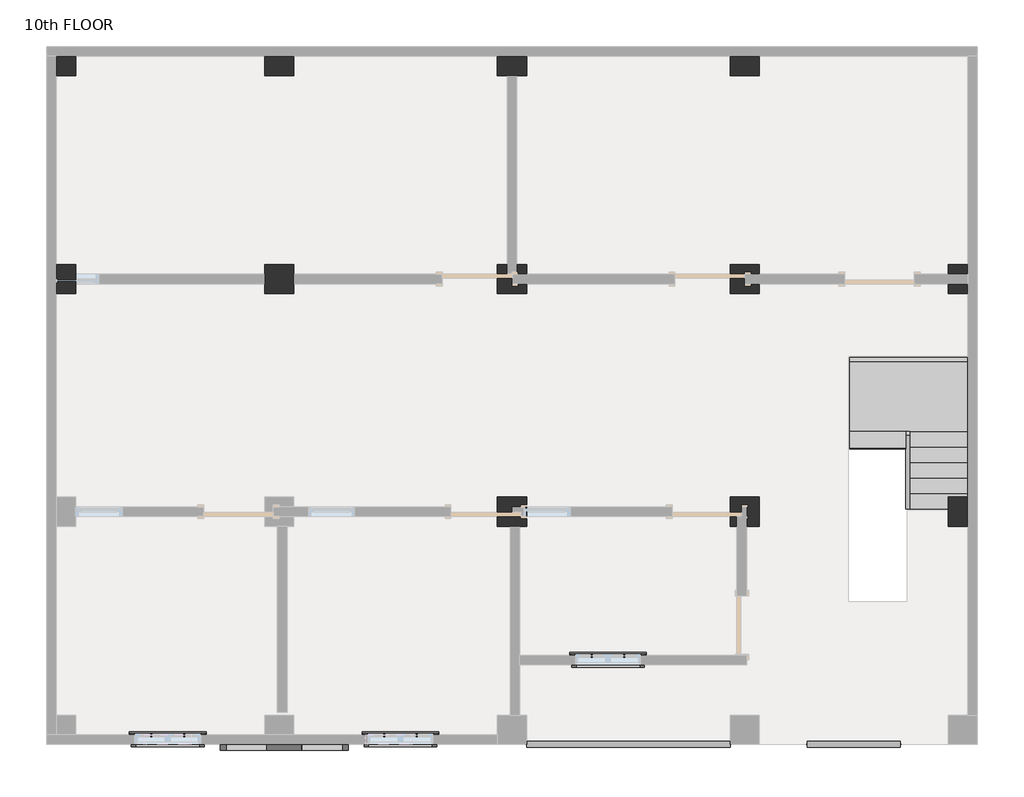
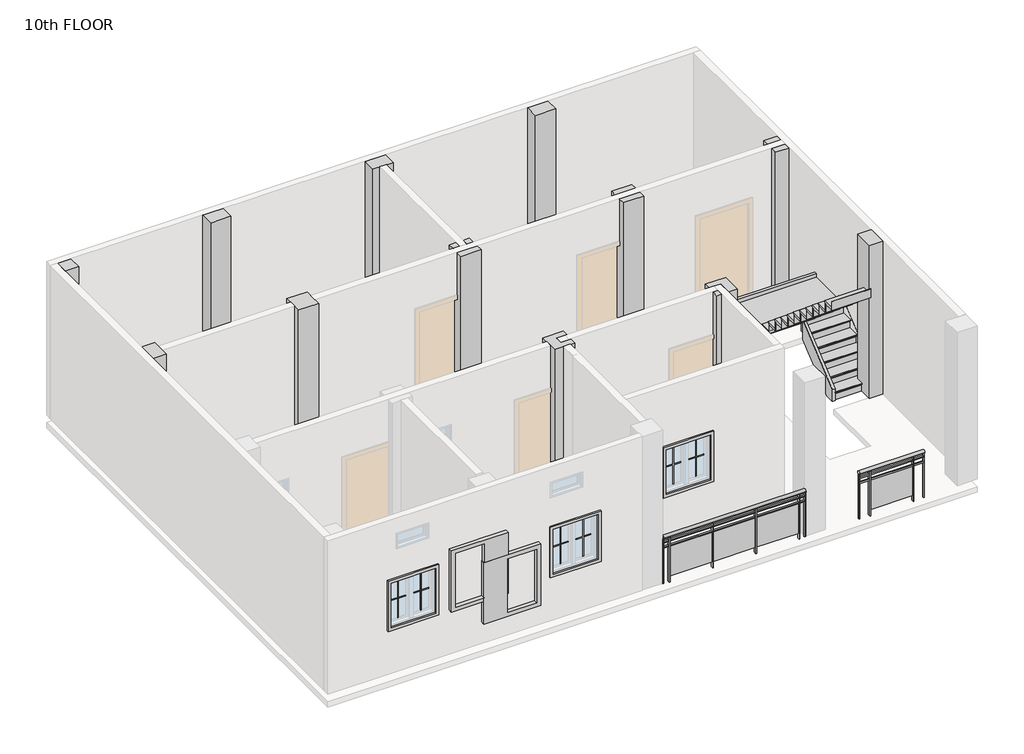
# One storey, part 2 of 2: 12 columns, 12 proxies, 4 members, 2 railings, 1 damper, 1 stair flight.
"""IFC4 building model written with IfcOpenShell, lengths in millimetres."""

from ifc_helpers import new_model, si_unit, point, frame, origin, place, context, project, spatial, polyline, ellipse_curve, trimmed, outline, extrude, faceted_brep, transform, mapped, element, save
from ifc_brep_helpers import plane_surface, extruded_surface, advanced_brep
from components import muntin_pattern_2x2_muntin_pattern_2x2_b3fe6957, muntin_pattern_2x2_muntin_pattern_2x2_3e0ecaf2, trim_window_exterior_flat_with_sill_41619996, trim_window_interior_flat_picture_frame_51c85655, duct_accessories_3_duct_accessories_1_969fcb05, stair_flight_e7bd6350

model = new_model("IFC4")

# Units and contexts
model_context = context("Model", 3, world=origin())
ifc_project = project(units=[si_unit("LENGTHUNIT", "METRE", prefix="MILLI")], contexts=[model_context])

# Site, building, storey
site = spatial("IfcSite", under=ifc_project)
building = spatial("IfcBuilding", under=site)
storey = spatial("IfcBuildingStorey", under=building, Name="10th FLOOR", Elevation=30327.6)

# Proxies
placement = place(None, origin())
muntin_pattern_2x2_muntin_pattern_2x2_shape = muntin_pattern_2x2_muntin_pattern_2x2_b3fe6957(model_context)
element("IfcBuildingElementProxy", 1, Name="Muntin Pattern_2x2 : Muntin Pattern_2x2", ObjectType="Muntin Pattern_2x2 : Muntin Pattern_2x2", at=placement, inside=storey, context=model_context, shape_type="MappedRepresentation", body=[
    mapped(muntin_pattern_2x2_muntin_pattern_2x2_shape, transform((-14441.409625, -253.8184478, 31311.85), x_axis=(1.0, 0.0, 0.0), y_axis=(0.0, 1.0, 0.0), z_axis=(0.0, 0.0, 1.0))),
])
element("IfcBuildingElementProxy", 2, Name="Muntin Pattern_2x2 : Muntin Pattern_2x2", ObjectType="Muntin Pattern_2x2 : Muntin Pattern_2x2", at=placement, inside=storey, context=model_context, shape_type="MappedRepresentation", body=[
    mapped(muntin_pattern_2x2_muntin_pattern_2x2_shape, transform((-11393.409625, -253.8184478, 31311.85), x_axis=(1.0, 0.0, 0.0), y_axis=(0.0, 1.0, 0.0), z_axis=(0.0, 0.0, 1.0))),
])
element("IfcBuildingElementProxy", 3, Name="Muntin Pattern_2x2 : Muntin Pattern_2x2", ObjectType="Muntin Pattern_2x2 : Muntin Pattern_2x2", at=placement, inside=storey, context=model_context, shape_type="MappedRepresentation", body=[
    mapped(muntin_pattern_2x2_muntin_pattern_2x2_shape, transform((-8675.609625, 787.5815522, 31311.85), x_axis=(1.0, 0.0, 0.0), y_axis=(0.0, 1.0, 0.0), z_axis=(0.0, 0.0, 1.0))),
])
muntin_pattern_2x2_muntin_pattern_2x2_2_shape = muntin_pattern_2x2_muntin_pattern_2x2_3e0ecaf2(model_context)
element("IfcBuildingElementProxy", 4, Name="Muntin Pattern_2x2 : Muntin Pattern_2x2", ObjectType="Muntin Pattern_2x2 : Muntin Pattern_2x2", at=placement, inside=storey, context=model_context, shape_type="MappedRepresentation", body=[
    mapped(muntin_pattern_2x2_muntin_pattern_2x2_2_shape, transform((-14012.784625, -253.8184478, 31311.85), x_axis=(-1.0, 0.0, 0.0), y_axis=(0.0, -1.0, 0.0), z_axis=(0.0, 0.0, 1.0))),
])
element("IfcBuildingElementProxy", 5, Name="Muntin Pattern_2x2 : Muntin Pattern_2x2", ObjectType="Muntin Pattern_2x2 : Muntin Pattern_2x2", at=placement, inside=storey, context=model_context, shape_type="MappedRepresentation", body=[
    mapped(muntin_pattern_2x2_muntin_pattern_2x2_2_shape, transform((-10964.784625, -253.8184478, 31311.85), x_axis=(-1.0, 0.0, 0.0), y_axis=(0.0, -1.0, 0.0), z_axis=(0.0, 0.0, 1.0))),
])
element("IfcBuildingElementProxy", 6, Name="Muntin Pattern_2x2 : Muntin Pattern_2x2", ObjectType="Muntin Pattern_2x2 : Muntin Pattern_2x2", at=placement, inside=storey, context=model_context, shape_type="MappedRepresentation", body=[
    mapped(muntin_pattern_2x2_muntin_pattern_2x2_2_shape, transform((-8246.984625, 787.5815522, 31311.85), x_axis=(-1.0, 0.0, 0.0), y_axis=(0.0, -1.0, 0.0), z_axis=(0.0, 0.0, 1.0))),
])
trim_window_exterior_flat_with_sill_shape = trim_window_exterior_flat_with_sill_41619996(model_context)
element("IfcBuildingElementProxy", 7, Name="Trim-Window-Exterior-Flat : with Sill", ObjectType="Trim-Window-Exterior-Flat : with Sill", at=placement, inside=storey, context=model_context, shape_type="MappedRepresentation", body=[
    mapped(trim_window_exterior_flat_with_sill_shape, transform((-14227.097125, -244.2934478, 32156.4), x_axis=(-1.0, 0.0, 0.0), y_axis=(0.0, 0.0, 1.0), z_axis=(0.0, 1.0, 0.0))),
])
element("IfcBuildingElementProxy", 8, Name="Trim-Window-Exterior-Flat : with Sill", ObjectType="Trim-Window-Exterior-Flat : with Sill", at=placement, inside=storey, context=model_context, shape_type="MappedRepresentation", body=[
    mapped(trim_window_exterior_flat_with_sill_shape, transform((-11179.097125, -244.2934478, 32156.4), x_axis=(-1.0, 0.0, 0.0), y_axis=(0.0, 0.0, 1.0), z_axis=(0.0, 1.0, 0.0))),
])
element("IfcBuildingElementProxy", 9, Name="Trim-Window-Exterior-Flat : with Sill", ObjectType="Trim-Window-Exterior-Flat : with Sill", at=placement, inside=storey, context=model_context, shape_type="MappedRepresentation", body=[
    mapped(trim_window_exterior_flat_with_sill_shape, transform((-8461.297125, 797.1065522, 32156.4), x_axis=(-1.0, 0.0, 0.0), y_axis=(0.0, 0.0, 1.0), z_axis=(0.0, 1.0, 0.0))),
])
trim_window_interior_flat_picture_frame_shape = trim_window_interior_flat_picture_frame_51c85655(model_context)
element("IfcBuildingElementProxy", 10, Name="Trim-Window-Interior-Flat : Picture Frame", ObjectType="Trim-Window-Interior-Flat : Picture Frame", at=placement, inside=storey, context=model_context, shape_type="MappedRepresentation", body=[
    mapped(trim_window_interior_flat_picture_frame_shape, transform((-14227.097125, -371.2934478, 32156.4), x_axis=(1.0, 0.0, 0.0), y_axis=(0.0, 0.0, 1.0), z_axis=(0.0, -1.0, 0.0))),
])
element("IfcBuildingElementProxy", 11, Name="Trim-Window-Interior-Flat : Picture Frame", ObjectType="Trim-Window-Interior-Flat : Picture Frame", at=placement, inside=storey, context=model_context, shape_type="MappedRepresentation", body=[
    mapped(trim_window_interior_flat_picture_frame_shape, transform((-11179.097125, -371.2934478, 32156.4), x_axis=(1.0, 0.0, 0.0), y_axis=(0.0, 0.0, 1.0), z_axis=(0.0, -1.0, 0.0))),
])
element("IfcBuildingElementProxy", 12, Name="Trim-Window-Interior-Flat : Picture Frame", ObjectType="Trim-Window-Interior-Flat : Picture Frame", at=placement, inside=storey, context=model_context, shape_type="MappedRepresentation", body=[
    mapped(trim_window_interior_flat_picture_frame_shape, transform((-8461.297125, 670.1065522, 32156.4), x_axis=(1.0, 0.0, 0.0), y_axis=(0.0, 0.0, 1.0), z_axis=(0.0, -1.0, 0.0))),
])

# Columns
element("IfcColumn", 13, ObjectType="column family : column family", at=placement, inside=storey, context=model_context, shape_type="SweptSolid", body=[
    extrude(outline(polyline([(-15433.597125, 8645.7065522), (-15433.597125, 8391.7065522), (-15687.597125, 8391.7065522), (-15687.597125, 8645.7065522), (-15433.597125, 8645.7065522)])), frame((0.0, 0.0, 30332.6), z_axis=(0.0, 0.0, 1.0), x_axis=(1.0, 0.0, 0.0)), (0.0, 0.0, 1.0), 3038.0),
])
element("IfcColumn", 14, ObjectType="column family : column family", at=placement, inside=storey, context=model_context, shape_type="SweptSolid", body=[
    extrude(outline(polyline([(-12576.097125, 5915.2065522), (-12576.097125, 5534.2065522), (-12957.097125, 5534.2065522), (-12957.097125, 5915.2065522), (-12576.097125, 5915.2065522)])), frame((0.0, 0.0, 30332.6), z_axis=(0.0, 0.0, 1.0), x_axis=(1.0, 0.0, 0.0)), (0.0, 0.0, 1.0), 3038.0),
])
element("IfcColumn", 15, ObjectType="column family : column family", at=placement, inside=storey, context=model_context, shape_type="Brep", body=[
    faceted_brep([(-9655.097125, 5915.2065522, 30332.6), (-9528.097125, 5915.2065522, 30332.6), (-9528.097125, 5788.2065522, 30332.6), (-9655.097125, 5788.2065522, 30332.6), (-9528.097125, 5915.2065522, 33370.6), (-9655.097125, 5915.2065522, 33370.6), (-9655.097125, 5788.2065522, 33370.6), (-9528.097125, 5788.2065522, 33370.6)], [[[0, 1, 2, 3]], [[4, 5, 6, 7]], [[0, 3, 6, 5]], [[4, 1, 0, 5]], [[3, 2, 7, 6]], [[1, 4, 7, 2]]]),
    faceted_brep([(-9528.097125, 5534.2065522, 33370.6), (-9528.097125, 5534.2065522, 30332.6), (-9528.097125, 5661.2065522, 30332.6), (-9528.097125, 5661.2065522, 33370.6), (-9909.097125, 5534.2065522, 30332.6), (-9909.097125, 5534.2065522, 33370.6), (-9909.097125, 5915.2065522, 30332.6), (-9909.097125, 5661.2065522, 33370.6), (-9909.097125, 5661.2065522, 32461.2), (-9909.097125, 5788.2065522, 32461.2), (-9909.097125, 5788.2065522, 33370.6), (-9909.097125, 5915.2065522, 33370.6), (-9782.097125, 5915.2065522, 33370.6), (-9782.097125, 5915.2065522, 30332.6), (-9782.097125, 5788.2065522, 30332.6), (-9782.097125, 5788.2065522, 33370.6), (-9782.097125, 5788.2065522, 32461.2), (-9718.597125, 5788.2065522, 30332.6), (-9718.597125, 5788.2065522, 32461.2), (-9718.597125, 5661.2065522, 30332.6), (-9718.597125, 5661.2065522, 32461.2)], [[[0, 1, 2, 3]], [[4, 1, 0, 5]], [[6, 4, 5, 7, 8, 9, 10, 11]], [[6, 11, 12, 13]], [[14, 13, 12, 15, 16]], [[17, 14, 16, 18]], [[19, 20, 8, 7, 3, 2]], [[1, 4, 6, 13, 14, 17, 19, 2]], [[5, 0, 3, 7]], [[12, 11, 10, 15]], [[9, 16, 15, 10]], [[18, 20, 19, 17]], [[20, 18, 16, 9, 8]]]),
])
element("IfcColumn", 16, ObjectType="column family : column family", at=placement, inside=storey, context=model_context, shape_type="Brep", body=[
    faceted_brep([(-6480.097125, 5534.2065522, 30332.6), (-6861.097125, 5534.2065522, 30332.6), (-6861.097125, 5915.2065522, 30332.6), (-6480.097125, 5915.2065522, 30332.6), (-6480.097125, 5788.2065522, 30332.6), (-6670.597125, 5788.2065522, 30332.6), (-6670.597125, 5661.2065522, 30332.6), (-6480.097125, 5661.2065522, 30332.6), (-6480.097125, 5534.2065522, 33370.6), (-6480.097125, 5661.2065522, 33370.6), (-6861.097125, 5534.2065522, 33370.6), (-6861.097125, 5661.2065522, 33370.6), (-6861.097125, 5661.2065522, 32461.2), (-6861.097125, 5788.2065522, 32461.2), (-6861.097125, 5788.2065522, 33370.6), (-6861.097125, 5915.2065522, 33370.6), (-6480.097125, 5915.2065522, 33370.6), (-6670.597125, 5661.2065522, 32461.2), (-6670.597125, 5788.2065522, 32461.2), (-6480.097125, 5788.2065522, 33370.6)], [[[0, 1, 2, 3, 4, 5, 6, 7]], [[8, 0, 7, 9]], [[1, 0, 8, 10]], [[2, 1, 10, 11, 12, 13, 14, 15]], [[3, 2, 15, 16]], [[10, 8, 9, 11]], [[6, 17, 12, 11, 9, 7]], [[13, 18, 5, 4, 19, 14]], [[3, 16, 19, 4]], [[16, 15, 14, 19]], [[18, 17, 6, 5]], [[17, 18, 13, 12]]]),
])
element("IfcColumn", 17, ObjectType="column family : column family", at=placement, inside=storey, context=model_context, shape_type="Brep", body=[
    faceted_brep([(-6480.097125, 2867.2065522, 30332.6), (-6480.097125, 2486.2065522, 30332.6), (-6645.197125, 2486.2065522, 30332.6), (-6645.197125, 2740.2065522, 30332.6), (-6708.697125, 2740.2065522, 30332.6), (-6708.697125, 2613.2065522, 30332.6), (-6772.197125, 2613.2065522, 30332.6), (-6772.197125, 2486.2065522, 30332.6), (-6861.097125, 2486.2065522, 30332.6), (-6861.097125, 2867.2065522, 30332.6), (-6480.097125, 2867.2065522, 33370.6), (-6480.097125, 2486.2065522, 33370.6), (-6861.097125, 2486.2065522, 33370.6), (-6772.197125, 2486.2065522, 33370.6), (-6861.097125, 2613.2065522, 33370.6), (-6861.097125, 2613.2065522, 32461.2), (-6861.097125, 2740.2065522, 32461.2), (-6861.097125, 2740.2065522, 33370.6), (-6861.097125, 2867.2065522, 33370.6), (-6772.197125, 2740.2065522, 33370.6), (-6645.197125, 2740.2065522, 33370.6), (-6645.197125, 2486.2065522, 33370.6), (-6772.197125, 2613.2065522, 33370.6), (-6772.197125, 2613.2065522, 32461.2), (-6772.197125, 2740.2065522, 32461.2), (-6708.697125, 2613.2065522, 32461.2), (-6708.697125, 2740.2065522, 32461.2)], [[[0, 1, 2, 3, 4, 5, 6, 7, 8, 9]], [[1, 0, 10, 11]], [[12, 8, 7, 13]], [[9, 8, 12, 14, 15, 16, 17, 18]], [[0, 9, 18, 10]], [[11, 10, 18, 17, 19, 20, 21]], [[15, 14, 22, 23]], [[17, 16, 24, 19]], [[20, 3, 2, 21]], [[6, 23, 22, 13, 7]], [[14, 12, 13, 22]], [[1, 11, 21, 2]], [[15, 23, 24, 16]], [[25, 23, 6, 5]], [[23, 25, 26, 24]], [[26, 25, 5, 4]], [[24, 26, 4, 3, 20, 19]]]),
])
element("IfcColumn", 18, ObjectType="column family : column family", at=placement, inside=storey, context=model_context, shape_type="Brep", body=[
    faceted_brep([(-9528.097125, 2486.2065522, 30332.6), (-9909.097125, 2486.2065522, 30332.6), (-9909.097125, 2867.2065522, 30332.6), (-9528.097125, 2867.2065522, 30332.6), (-9528.097125, 2740.2065522, 30332.6), (-9566.197125, 2740.2065522, 30332.6), (-9718.597125, 2740.2065522, 30332.6), (-9718.597125, 2613.2065522, 30332.6), (-9566.197125, 2613.2065522, 30332.6), (-9528.097125, 2613.2065522, 30332.6), (-9528.097125, 2486.2065522, 33370.6), (-9528.097125, 2613.2065522, 30632.4), (-9528.097125, 2740.2065522, 30632.4), (-9528.097125, 2867.2065522, 33370.6), (-9528.097125, 2740.2065522, 33370.6), (-9528.097125, 2740.2065522, 32461.2), (-9528.097125, 2613.2065522, 32461.2), (-9528.097125, 2613.2065522, 33370.6), (-9909.097125, 2486.2065522, 33370.6), (-9909.097125, 2867.2065522, 33370.6), (-9566.197125, 2613.2065522, 33370.6), (-9718.597125, 2613.2065522, 33370.6), (-9718.597125, 2740.2065522, 33370.6), (-9566.197125, 2740.2065522, 33370.6), (-9566.197125, 2613.2065522, 32461.2), (-9566.197125, 2613.2065522, 30632.4), (-9566.197125, 2740.2065522, 30632.4), (-9566.197125, 2740.2065522, 32461.2)], [[[0, 1, 2, 3, 4, 5, 6, 7, 8, 9]], [[10, 0, 9, 11, 12, 4, 3, 13, 14, 15, 16, 17]], [[1, 0, 10, 18]], [[2, 1, 18, 19]], [[3, 2, 19, 13]], [[18, 10, 17, 20, 21, 22, 23, 14, 13, 19]], [[11, 9, 8, 7, 21, 20, 17, 16, 24, 25]], [[4, 12, 26, 27, 15, 14, 23, 22, 6, 5]], [[21, 7, 6, 22]], [[25, 24, 27, 26]], [[25, 26, 12, 11]], [[27, 24, 16, 15]]]),
])
element("IfcColumn", 19, ObjectType="column family : column family", at=placement, inside=storey, context=model_context, shape_type="SweptSolid", body=[
    extrude(outline(polyline([(-12576.097125, 8391.7065522), (-12957.097125, 8391.7065522), (-12957.097125, 8645.7065522), (-12576.097125, 8645.7065522), (-12576.097125, 8391.7065522)])), frame((0.0, 0.0, 30332.6), z_axis=(0.0, 0.0, 1.0), x_axis=(1.0, 0.0, 0.0)), (0.0, 0.0, 1.0), 3038.0),
])
element("IfcColumn", 20, ObjectType="column family : column family", at=placement, inside=storey, context=model_context, shape_type="SweptSolid", body=[
    extrude(outline(polyline([(-9528.097125, 8391.7065522), (-9909.097125, 8391.7065522), (-9909.097125, 8645.7065522), (-9528.097125, 8645.7065522), (-9528.097125, 8391.7065522)])), frame((0.0, 0.0, 30332.6), z_axis=(0.0, 0.0, 1.0), x_axis=(1.0, 0.0, 0.0)), (0.0, 0.0, 1.0), 3038.0),
])
element("IfcColumn", 21, ObjectType="column family : column family", at=placement, inside=storey, context=model_context, shape_type="SweptSolid", body=[
    extrude(outline(polyline([(-6480.097125, 8391.7065522), (-6861.097125, 8391.7065522), (-6861.097125, 8645.7065522), (-6480.097125, 8645.7065522), (-6480.097125, 8391.7065522)])), frame((0.0, 0.0, 30332.6), z_axis=(0.0, 0.0, 1.0), x_axis=(1.0, 0.0, 0.0)), (0.0, 0.0, 1.0), 3038.0),
])
element("IfcColumn", 22, ObjectType="column family : column family", at=placement, inside=storey, context=model_context, shape_type="SweptSolid", body=[
    extrude(outline(polyline([(-4003.597125, 5915.2065522), (-3749.597125, 5915.2065522), (-3749.597125, 5788.2065522), (-4003.597125, 5788.2065522), (-4003.597125, 5915.2065522)])), frame((0.0, 0.0, 30332.6), z_axis=(0.0, 0.0, 1.0), x_axis=(1.0, 0.0, 0.0)), (0.0, 0.0, 1.0), 3038.0),
    extrude(outline(polyline([(-3749.597125, 5534.2065522), (-4003.597125, 5534.2065522), (-4003.597125, 5661.2065522), (-3749.597125, 5661.2065522), (-3749.597125, 5534.2065522)])), frame((0.0, 0.0, 30332.6), z_axis=(0.0, 0.0, 1.0), x_axis=(1.0, 0.0, 0.0)), (0.0, 0.0, 1.0), 3038.0),
])
element("IfcColumn", 23, ObjectType="column family : column family", at=placement, inside=storey, context=model_context, shape_type="SweptSolid", body=[
    extrude(outline(polyline([(-4003.597125, 2486.2065522), (-4003.597125, 2867.2065522), (-3749.597125, 2867.2065522), (-3749.597125, 2486.2065522), (-4003.597125, 2486.2065522)])), frame((0.0, 0.0, 30332.6), z_axis=(0.0, 0.0, 1.0), x_axis=(1.0, 0.0, 0.0)), (0.0, 0.0, 1.0), 3038.0),
])
element("IfcColumn", 24, ObjectType="column family : column family", at=placement, inside=storey, context=model_context, shape_type="SweptSolid", body=[
    extrude(outline(polyline([(-15433.597125, 5915.2065522), (-15433.597125, 5534.2065522), (-15687.597125, 5534.2065522), (-15687.597125, 5915.2065522), (-15433.597125, 5915.2065522)])), frame((0.0, 0.0, 30332.6), z_axis=(0.0, 0.0, 1.0), x_axis=(1.0, 0.0, 0.0)), (0.0, 0.0, 1.0), 3038.0),
])

# Damper
duct_accessories_3_duct_accessories_1_shape = duct_accessories_3_duct_accessories_1_969fcb05(model_context)
element("IfcDamper", 25, ObjectType="Duct Accessories 3 : Duct Accessories 1", at=placement, inside=storey, context=model_context, shape_type="MappedRepresentation", body=[
    mapped(duct_accessories_3_duct_accessories_1_shape, transform((0.0, 0.0, 0.0), x_axis=(1.0, 0.0, 0.0), y_axis=(0.0, 1.0, 0.0), z_axis=(0.0, 0.0, 1.0))),
])

# Members
element("IfcMember", 26, ObjectType="Stringer - 2\" Width", at=placement, inside=storey, context=model_context, shape_type="SweptSolid", body=[
    extrude(outline(polyline([(2714.6319226, 30327.6), (2714.6319226, 30564.4438745), (3679.8319226, 31368.7772078), (3679.8319226, 30972.0165243), (2906.5320935, 30327.6), (2714.6319226, 30327.6)])), frame((-4563.0136682, 0.0, 0.0), z_axis=(1.0, 0.0, 0.0), x_axis=(0.0, 1.0, 0.0)), (0.0, 0.0, 1.0), 50.8),
])
element("IfcMember", 27, ObjectType="Stringer - 2\" Width", at=placement, inside=storey, context=model_context, shape_type="SweptSolid", body=[
    extrude(outline(polyline([(-4512.2136682, 3730.6319226), (-4512.2136682, 3679.8319226), (-4563.0136682, 3679.8319226), (-4563.0136682, 3730.6319226), (-4512.2136682, 3730.6319226)])), frame((0.0, 0.0, 31115.0), z_axis=(0.0, 0.0, 1.0), x_axis=(1.0, 0.0, 0.0)), (0.0, 0.0, 1.0), 304.8),
])
element("IfcMember", 28, ObjectType="Stringer - 2\" Width", at=placement, inside=storey, context=model_context, shape_type="SweptSolid", body=[
    extrude(outline(polyline([(2714.6319226, 30327.6), (2714.6319226, 30564.4438745), (3741.0592732, 31419.8), (4217.1720935, 31419.8), (2906.5320935, 30327.6), (2714.6319226, 30327.6)])), frame((-3749.597125, 0.0, 0.0), z_axis=(1.0, 0.0, 0.0), x_axis=(0.0, 1.0, 0.0)), (0.0, 0.0, 1.0), 50.8),
])
element("IfcMember", 29, ObjectType="Stringer - 2\" Width", at=placement, inside=storey, context=model_context, shape_type="SweptSolid", body=[
    extrude(outline(polyline([(-3698.797125, 4695.8319226), (-3698.797125, 4645.0319226), (-5295.0246464, 4645.0319226), (-5295.0246464, 4695.8319226), (-3698.797125, 4695.8319226)])), frame((0.0, 0.0, 31115.0), z_axis=(0.0, 0.0, 1.0), x_axis=(1.0, 0.0, 0.0)), (0.0, 0.0, 1.0), 304.8),
])

# Railings
element("IfcRailing", 30, ObjectType="Glass Panel - Bottom Fill", at=placement, inside=storey, context=model_context, shape_type="SolidModel", body=[
    advanced_brep(
    [(-9528.097125, -333.1934478, 31242.0), (-9528.097125, -409.3934478, 31242.0), (-6861.097125, -333.1934478, 31242.0), (-6861.097125, -409.3934478, 31242.0)],
    [
        (0, 1, ellipse_curve(frame((-9528.097125, -371.2934478, 31242.0), z_axis=(-1.0, 0.0, 0.0), x_axis=(0.0, -1.0, 0.0)), 38.1, 28.575)),
        (1, 0, ellipse_curve(frame((-9528.097125, -371.2934478, 31242.0), z_axis=(-1.0, 0.0, 0.0), x_axis=(0.0, -1.0, 0.0)), 38.1, 28.575)),
        (2, 3, ellipse_curve(frame((-6861.097125, -371.2934478, 31242.0), z_axis=(1.0, 0.0, 0.0), x_axis=(0.0, -1.0, 0.0)), 38.1, 28.575)),
        (3, 2, ellipse_curve(frame((-6861.097125, -371.2934478, 31242.0), z_axis=(1.0, 0.0, 0.0), x_axis=(0.0, -1.0, 0.0)), 38.1, 28.575)),
        (0, 2),
        (3, 1),
    ],
    [
        plane_surface(frame((-9528.097125, -371.2934478, 31242.0), z_axis=(-1.0, 0.0, 0.0), x_axis=(0.0, 1.0, 0.0))),
        plane_surface(frame((-6861.097125, -371.2934478, 31242.0), z_axis=(1.0, 0.0, 0.0), x_axis=(0.0, 1.0, 0.0))),
        extruded_surface(trimmed(ellipse_curve(frame((-6861.097125, -371.2934478, 31242.0), z_axis=(-1.0, 0.0, 0.0), x_axis=(0.0, -1.0, 0.0)), 38.1, 28.575), [point((-6861.097125, -333.1934478, 31242.0))], [point((-6861.097125, -409.3934478, 31242.0))], True, "CARTESIAN"), (-2667.0, 0.0, 0.0), 2667.0),
        extruded_surface(trimmed(ellipse_curve(frame((-6861.097125, -371.2934478, 31242.0), z_axis=(-1.0, 0.0, 0.0), x_axis=(0.0, -1.0, 0.0)), 38.1, 28.575), [point((-6861.097125, -409.3934478, 31242.0))], [point((-6861.097125, -333.1934478, 31242.0))], True, "CARTESIAN"), (-2667.0, 0.0, 0.0), 2667.0),
    ],
    [
        (0, [[1, 2]]),
        (1, [[3, 4]]),
        (2, [[-1, 5, -4, 6]]),
        (3, [[-2, -6, -3, -5]]),
    ],
),
    extrude(outline(polyline([(-9528.097125, -383.9934478), (-9528.097125, -358.5934478), (-6861.097125, -358.5934478), (-6861.097125, -383.9934478), (-9528.097125, -383.9934478)])), frame((0.0, 0.0, 31127.7), z_axis=(0.0, 0.0, 1.0), x_axis=(1.0, 0.0, 0.0)), (0.0, 0.0, 1.0), 25.4),
    extrude(outline(polyline([(-9528.097125, -383.9934478), (-9528.097125, -358.5934478), (-6861.097125, -358.5934478), (-6861.097125, -383.9934478), (-9528.097125, -383.9934478)])), frame((0.0, 0.0, 31026.1), z_axis=(0.0, 0.0, 1.0), x_axis=(1.0, 0.0, 0.0)), (0.0, 0.0, 1.0), 25.4),
    extrude(outline(polyline([(-6981.747125, -396.6934478), (-6981.747125, -345.8934478), (-6969.047125, -345.8934478), (-6969.047125, -396.6934478), (-6981.747125, -396.6934478)])), frame((0.0, 0.0, 30327.6), z_axis=(0.0, 0.0, 1.0), x_axis=(1.0, 0.0, 0.0)), (0.0, 0.0, 1.0), 885.6788223),
    extrude(outline(polyline([(-7788.197125, -364.7582908), (-6975.397125, -364.7582908), (-6975.397125, -371.1082908), (-7788.197125, -371.1082908), (-7788.197125, -364.7582908)])), frame((0.0, 0.0, 30429.2), z_axis=(0.0, 0.0, 1.0), x_axis=(1.0, 0.0, 0.0)), (0.0, 0.0, 1.0), 596.9),
    extrude(outline(polyline([(-7794.547125, -396.6934478), (-7794.547125, -345.8934478), (-7781.847125, -345.8934478), (-7781.847125, -396.6934478), (-7794.547125, -396.6934478)])), frame((0.0, 0.0, 30327.6), z_axis=(0.0, 0.0, 1.0), x_axis=(1.0, 0.0, 0.0)), (0.0, 0.0, 1.0), 885.6788223),
    extrude(outline(polyline([(-8600.997125, -364.7582908), (-7788.197125, -364.7582908), (-7788.197125, -371.1082908), (-8600.997125, -371.1082908), (-8600.997125, -364.7582908)])), frame((0.0, 0.0, 30429.2), z_axis=(0.0, 0.0, 1.0), x_axis=(1.0, 0.0, 0.0)), (0.0, 0.0, 1.0), 596.9),
    extrude(outline(polyline([(-8607.347125, -396.6934478), (-8607.347125, -345.8934478), (-8594.647125, -345.8934478), (-8594.647125, -396.6934478), (-8607.347125, -396.6934478)])), frame((0.0, 0.0, 30327.6), z_axis=(0.0, 0.0, 1.0), x_axis=(1.0, 0.0, 0.0)), (0.0, 0.0, 1.0), 885.6788223),
    extrude(outline(polyline([(-9413.797125, -364.7582908), (-8600.997125, -364.7582908), (-8600.997125, -371.1082908), (-9413.797125, -371.1082908), (-9413.797125, -364.7582908)])), frame((0.0, 0.0, 30429.2), z_axis=(0.0, 0.0, 1.0), x_axis=(1.0, 0.0, 0.0)), (0.0, 0.0, 1.0), 596.9),
    extrude(outline(polyline([(-9420.147125, -396.6934478), (-9420.147125, -345.8934478), (-9407.447125, -345.8934478), (-9407.447125, -396.6934478), (-9420.147125, -396.6934478)])), frame((0.0, 0.0, 30327.6), z_axis=(0.0, 0.0, 1.0), x_axis=(1.0, 0.0, 0.0)), (0.0, 0.0, 1.0), 885.6788223),
    extrude(outline(polyline([(-6873.797125, -380.8184478), (-6873.797125, -361.7684478), (-6854.747125, -361.7684478), (-6854.747125, -380.8184478), (-6873.797125, -380.8184478)])), frame((0.0, 0.0, 30327.6), z_axis=(0.0, 0.0, 1.0), x_axis=(1.0, 0.0, 0.0)), (0.0, 0.0, 1.0), 885.6788223),
    extrude(outline(polyline([(-9534.447125, -380.8184478), (-9534.447125, -361.7684478), (-9515.397125, -361.7684478), (-9515.397125, -380.8184478), (-9534.447125, -380.8184478)])), frame((0.0, 0.0, 30327.6), z_axis=(0.0, 0.0, 1.0), x_axis=(1.0, 0.0, 0.0)), (0.0, 0.0, 1.0), 885.6788223),
])
element("IfcRailing", 31, ObjectType="Glass Panel - Bottom Fill", at=placement, inside=storey, context=model_context, shape_type="SolidModel", body=[
    advanced_brep(
    [(-5851.447125, -333.1934478, 31242.0), (-5851.447125, -409.3934478, 31242.0), (-4632.247125, -333.1934478, 31242.0), (-4632.247125, -409.3934478, 31242.0)],
    [
        (0, 1, ellipse_curve(frame((-5851.447125, -371.2934478, 31242.0), z_axis=(-1.0, 0.0, 0.0), x_axis=(0.0, -1.0, 0.0)), 38.1, 28.575)),
        (1, 0, ellipse_curve(frame((-5851.447125, -371.2934478, 31242.0), z_axis=(-1.0, 0.0, 0.0), x_axis=(0.0, -1.0, 0.0)), 38.1, 28.575)),
        (2, 3, ellipse_curve(frame((-4632.247125, -371.2934478, 31242.0), z_axis=(1.0, 0.0, 0.0), x_axis=(0.0, -1.0, 0.0)), 38.1, 28.575)),
        (3, 2, ellipse_curve(frame((-4632.247125, -371.2934478, 31242.0), z_axis=(1.0, 0.0, 0.0), x_axis=(0.0, -1.0, 0.0)), 38.1, 28.575)),
        (0, 2),
        (3, 1),
    ],
    [
        plane_surface(frame((-5851.447125, -371.2934478, 31242.0), z_axis=(-1.0, 0.0, 0.0), x_axis=(0.0, 1.0, 0.0))),
        plane_surface(frame((-4632.247125, -371.2934478, 31242.0), z_axis=(1.0, 0.0, 0.0), x_axis=(0.0, 1.0, 0.0))),
        extruded_surface(trimmed(ellipse_curve(frame((-4632.247125, -371.2934478, 31242.0), z_axis=(-1.0, 0.0, 0.0), x_axis=(0.0, -1.0, 0.0)), 38.1, 28.575), [point((-4632.247125, -333.1934478, 31242.0))], [point((-4632.247125, -409.3934478, 31242.0))], True, "CARTESIAN"), (-1219.1999999999998, 0.0, 0.0), 1219.1999999999998),
        extruded_surface(trimmed(ellipse_curve(frame((-4632.247125, -371.2934478, 31242.0), z_axis=(-1.0, 0.0, 0.0), x_axis=(0.0, -1.0, 0.0)), 38.1, 28.575), [point((-4632.247125, -409.3934478, 31242.0))], [point((-4632.247125, -333.1934478, 31242.0))], True, "CARTESIAN"), (-1219.1999999999998, 0.0, 0.0), 1219.1999999999998),
    ],
    [
        (0, [[1, 2]]),
        (1, [[3, 4]]),
        (2, [[-1, 5, -4, 6]]),
        (3, [[-2, -6, -3, -5]]),
    ],
),
    extrude(outline(polyline([(-5851.447125, -383.9934478), (-5851.447125, -358.5934478), (-4632.247125, -358.5934478), (-4632.247125, -383.9934478), (-5851.447125, -383.9934478)])), frame((0.0, 0.0, 31127.7), z_axis=(0.0, 0.0, 1.0), x_axis=(1.0, 0.0, 0.0)), (0.0, 0.0, 1.0), 25.4),
    extrude(outline(polyline([(-5851.447125, -383.9934478), (-5851.447125, -358.5934478), (-4632.247125, -358.5934478), (-4632.247125, -383.9934478), (-5851.447125, -383.9934478)])), frame((0.0, 0.0, 31026.1), z_axis=(0.0, 0.0, 1.0), x_axis=(1.0, 0.0, 0.0)), (0.0, 0.0, 1.0), 25.4),
    extrude(outline(polyline([(-4841.797125, -396.6934478), (-4841.797125, -345.8934478), (-4829.097125, -345.8934478), (-4829.097125, -396.6934478), (-4841.797125, -396.6934478)])), frame((0.0, 0.0, 30327.6), z_axis=(0.0, 0.0, 1.0), x_axis=(1.0, 0.0, 0.0)), (0.0, 0.0, 1.0), 885.6788223),
    extrude(outline(polyline([(-5648.247125, -364.7582908), (-4835.447125, -364.7582908), (-4835.447125, -371.1082908), (-5648.247125, -371.1082908), (-5648.247125, -364.7582908)])), frame((0.0, 0.0, 30429.2), z_axis=(0.0, 0.0, 1.0), x_axis=(1.0, 0.0, 0.0)), (0.0, 0.0, 1.0), 596.9),
    extrude(outline(polyline([(-5654.597125, -396.6934478), (-5654.597125, -345.8934478), (-5641.897125, -345.8934478), (-5641.897125, -396.6934478), (-5654.597125, -396.6934478)])), frame((0.0, 0.0, 30327.6), z_axis=(0.0, 0.0, 1.0), x_axis=(1.0, 0.0, 0.0)), (0.0, 0.0, 1.0), 885.6788223),
    extrude(outline(polyline([(-4644.947125, -380.8184478), (-4644.947125, -361.7684478), (-4625.897125, -361.7684478), (-4625.897125, -380.8184478), (-4644.947125, -380.8184478)])), frame((0.0, 0.0, 30327.6), z_axis=(0.0, 0.0, 1.0), x_axis=(1.0, 0.0, 0.0)), (0.0, 0.0, 1.0), 885.6788223),
    extrude(outline(polyline([(-5857.797125, -380.8184478), (-5857.797125, -361.7684478), (-5838.747125, -361.7684478), (-5838.747125, -380.8184478), (-5857.797125, -380.8184478)])), frame((0.0, 0.0, 30327.6), z_axis=(0.0, 0.0, 1.0), x_axis=(1.0, 0.0, 0.0)), (0.0, 0.0, 1.0), 885.6788223),
])

# Stair flight
stair_flight_shape = stair_flight_e7bd6350(model_context)
element("IfcStairFlight", 32, ObjectType="2\" Tread 1\" Nosing 1/4\" Riser", at=placement, inside=storey, context=model_context, shape_type="MappedRepresentation", body=[
    mapped(stair_flight_shape, transform((0.0, 0.0, 0.0), x_axis=(1.0, 0.0, 0.0), y_axis=(0.0, 1.0, 0.0), z_axis=(0.0, 0.0, 1.0))),
])

save(model, "model.ifc")

# Revit data of these elements
# Type "Muntin Pattern_2x2 : Muntin Pattern_2x2"
#   Width [instance default] = 4' - 0"
#   Thickness = 0' - 0 1/2"
#   Height [instance default] = 4' - 0"
#   Distance = 0' - 0 3/4"
#   Interior Material [instance default] = none
#   Exterior Material [instance default] = none
#   Default Elevation = 0
# Type "Trim-Window-Exterior-Flat : with Sill"
#   Trim Width = 0' - 2 1/4"
#   Trim Thickness_Picture Frame = 0' - 1 1/4"
#   Trim Thickness_with Sill = 0' - 0 3/4"
#   Sill Thickness = 0' - 1 1/4"
#   Opening Width [instance default] = 2' - 0"
#   Opening Height [instance default] = 3' - 0"
#   Default Elevation = 4' - 0"
#   Sill = yes
#   Picture Frame = no
#   Trim Material [instance default] = none
# Type "Trim-Window-Interior-Flat : Picture Frame"
#   Trim Thickness_Picture Frame = 0' - 1 1/4"
#   Trim Width = 0' - 2 1/4"
#   Trim Thickness_with Sill = 0' - 0 3/4"
#   Sill Thickness = 0' - 1 1/4"
#   Opening Width [instance default] = 2' - 0"
#   Opening Height [instance default] = 3' - 0"
#   Default Elevation = 4' - 0"
#   Sill = no
#   Picture Frame = yes
#   Trim Material [instance default] = none
# Type "column family : column family"
#   w2 [instance default] = 0' - 9.88189"
#   w1 [instance default] = 0' - 9.01575"
#   Depth = 1' - 11.62205"
#   Width = 1' - 11.62205"
# Type "Glass Panel - Bottom Fill"
#   Assembly Code = "C2010400"
#   built-in parameter 1008612 = 0.0416667 (stored number, unit not read)
#   built-in parameter 1008611 = 0.0416667 (stored number, unit not read)
#   built-in parameter 1008609 = 0.333333 (stored number, unit not read)
#   built-in parameter 1008604 = 0.166667 (stored number, unit not read)
#   built-in parameter 1008603 = 0.166667 (stored number, unit not read)
#   Railing Height = 3' - 0"
#   built-in parameter 1008630 = 2
#   built-in parameter 1008610 = 2
#   built-in parameter 1008618 = Baluster - Square : 3/4"
# Elements 1, 2, 3, 4, 5, 6 (IfcBuildingElementProxy, "Muntin Pattern_2x2 : Muntin Pattern_2x2")
#   Width = 0' - 11 5/8"
#   Height = 2' - 6 1/2"
#   Interior Material = Wood - Stained
#   Exterior Material = Clad - White
#   Phase Created = New Construction
#   Materials on its faces: "Clad - White", "Wood - Stained"
# Elements 7, 8, 9 (IfcBuildingElementProxy, "Trim-Window-Exterior-Flat : with Sill")
#   Opening Width = 2' - 10"
#   Opening Height = 3' - 0"
#   Trim Material = Clad - White
#   Phase Created = New Construction
#   Materials on its faces: "Clad - White"
# Elements 10, 11, 12 (IfcBuildingElementProxy, "Trim-Window-Interior-Flat : Picture Frame")
#   Opening Width = 2' - 10"
#   Opening Height = 3' - 0"
#   Trim Material = Wood - Stained
#   Phase Created = New Construction
#   Materials on its faces: "Wood - Stained"
# Elements 13, 14, 15, 19, 20, 21 (IfcColumn, "column family : column family")
#   w2 = 1' - 3"
#   w1 = 1' - 3"
#   Phase Created = New Construction
#   Materials on its faces: "Default Wall"
# Elements 16, 22, 23 (IfcColumn, "column family : column family")
#   w2 = 1' - 3"
#   w1 = 1' - 3"
#   Phase Created = New Construction
#   Materials on its faces: "grey", "Default Wall"
# Elements 17, 18 (IfcColumn, "column family : column family")
#   w2 = 1' - 3"
#   w1 = 1' - 3"
#   Phase Created = New Construction
#   Materials on its faces: "Default Wall", "inside wall"
# Element 24 (IfcColumn, "column family : column family")
#   w2 = 1' - 3"
#   w1 = 1' - 3"
#   Phase Created = New Construction
#   Materials on its faces: "inside wall", "Default Wall"
# Element 25 (IfcDamper, "Duct Accessories 3 : Duct Accessories 1")
#   Mark = "3"
#   Phase Created = New Construction
#   Materials on its faces: "border"
# Elements 26, 27, 28, 29 (IfcMember, "Stringer - 2\" Width")
#   Phase Created = New Construction
# Elements 30, 31 (IfcRailing, "Glass Panel - Bottom Fill")
#   Phase Created = New Construction
#   Materials on its faces: "Glass"
# Element 32 (IfcStairFlight, "2\" Tread 1\" Nosing 1/4\" Riser")
#   Phase Created = New Construction
# Materials
#   "Clad - White": class "Wood", colour RGB 242 242 238, transparency 0, Cost = 0
#   "Wood - Stained": class "Wood", colour RGB 224 178 126, transparency 0, Cost = 0
#   "Default Wall": colour RGB 128 128 128, transparency 0, Cost = 0
#   "grey": class "Generic", colour RGB 80 80 80, transparency 0, Cost = 0
#   "inside wall": class "Generic", colour RGB 199 224 95, transparency 0, Cost = 0
#   "border": class "Generic", colour RGB 144 144 144, transparency 0, Cost = 0
#   "Glass": class "Glass", colour RGB 0 128 192, transparency 0.75, Description = "Soda Lime Glass", Cost = 0
